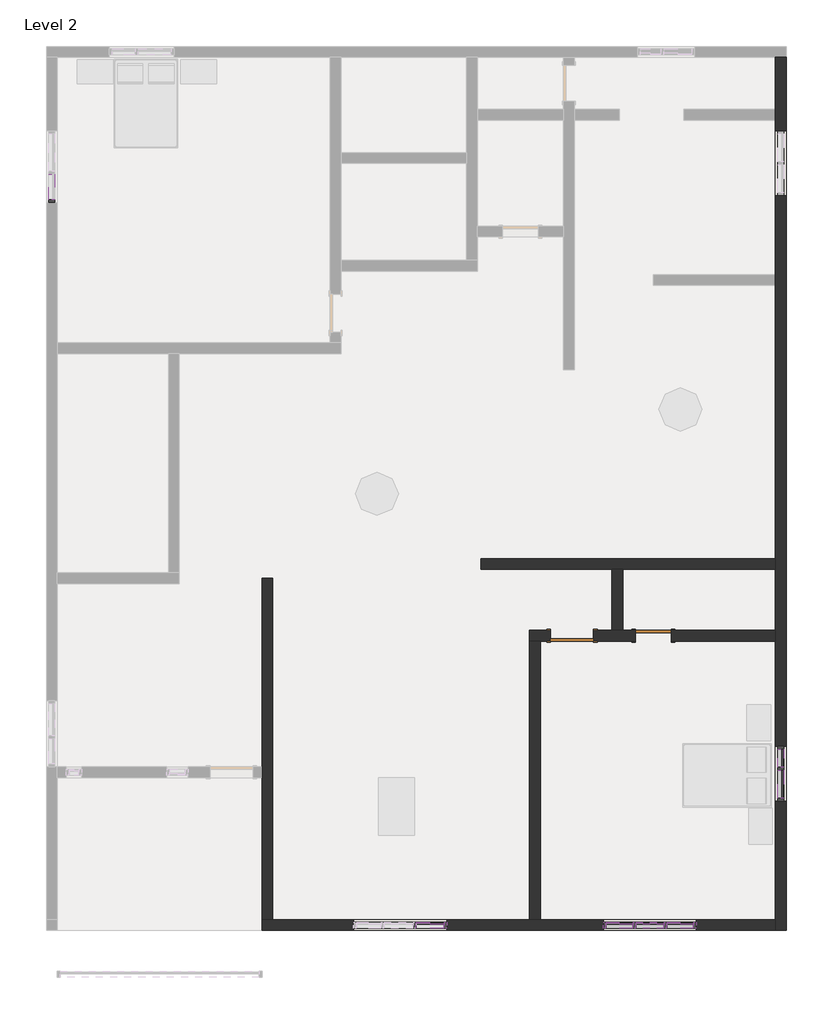
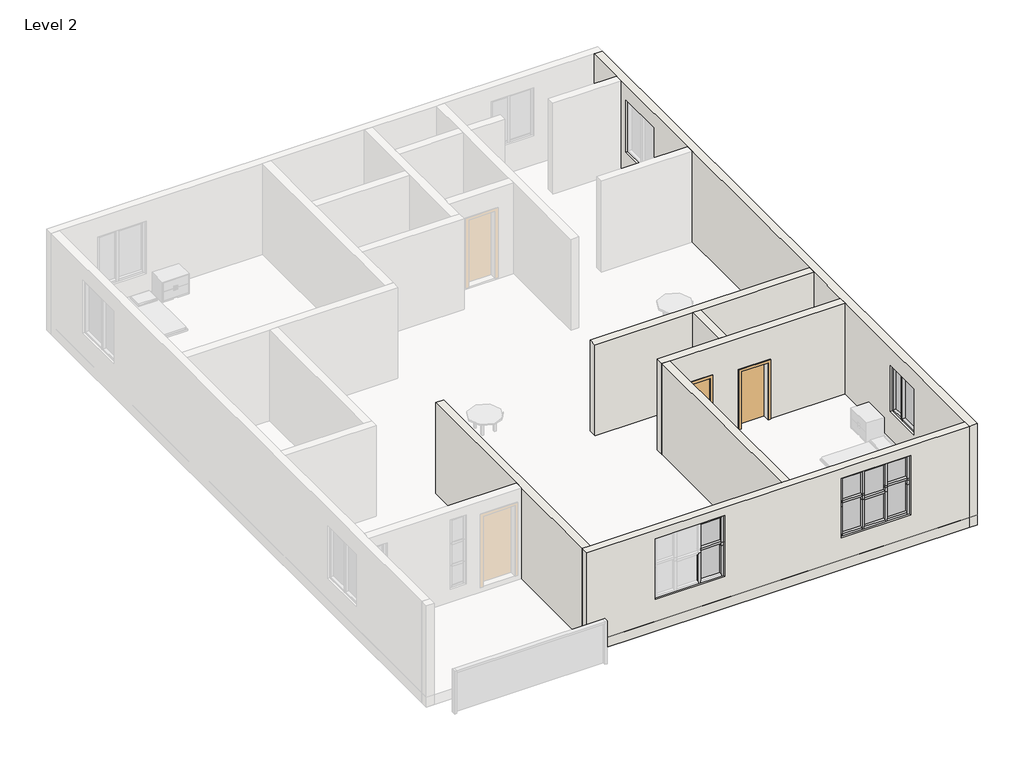
# One storey, part 2 of 3: 40 members, 10 plates, 7 walls, 2 doors.
"""IFC4 building model written with IfcOpenShell, lengths in millimetres."""

from ifc_helpers import new_model, si_unit, frame, origin, place, context, project, spatial, polyline, outline, extrude, faceted_brep, transform, mapped, element, save
from components import door_a1484949, door_0ca8825f, member_6f432376, member_6103f85b, member_a400357f, member_86293703, member_dffdf235, member_e5d39754, member_4dfd3f86, member_6a2a75bf, member_411778f3, member_a8e3eee7, member_06e32611, member_a86422a6, member_06be906d, member_67d1cd44, member_7190e7de, member_9cc26bde, member_6a93b315, member_fb13da3b, member_5b006e0e, member_8ea47e38, member_29dce480, member_81de2198, member_b315899a, system_panel_glazed_958ccbb4, system_panel_glazed_a29d5ab1, system_panel_glazed_48a86efd, system_panel_glazed_6d48a8a8, system_panel_glazed_893369a6, system_panel_glazed_ba2d6641, system_panel_glazed_82992491, system_panel_glazed_5721f284, system_panel_glazed_0c2a6c90, system_panel_glazed_e4ad360d

model = new_model("IFC4")

# Units and contexts
model_context = context("Model", 3, world=origin())
ifc_project = project(units=[si_unit("LENGTHUNIT", "METRE", prefix="MILLI")], contexts=[model_context])

# Site, building, storey
site = spatial("IfcSite", under=ifc_project)
building = spatial("IfcBuilding", under=site)
storey = spatial("IfcBuildingStorey", under=building, Name="Level 2", Elevation=3048.0)

# Doors
placement = place(None, origin())
door_shape = door_a1484949(model_context)
element("IfcDoor", 1, ObjectType="Single-Flush : 30\" x 80\"", at=placement, inside=storey, context=model_context, shape_type="MappedRepresentation", body=[
    mapped(door_shape, transform((-6207.9702714, -5339.3383903, 3048.0), x_axis=(1.0, 0.0, 0.0), y_axis=(0.0, 1.0, 0.0), z_axis=(0.0, 0.0, 1.0))),
])
door_2_shape = door_0ca8825f(model_context)
element("IfcDoor", 2, ObjectType="Single-Flush : 36\" x 84\"", at=placement, inside=storey, context=model_context, shape_type="MappedRepresentation", body=[
    mapped(door_2_shape, transform((-7935.1702714, -5339.3383903, 3048.0), x_axis=(-1.0, 0.0, 0.0), y_axis=(0.0, -1.0, 0.0), z_axis=(0.0, 0.0, 1.0))),
])

# Members
member_shape = member_6f432376(model_context)
element("IfcMember", 3, ObjectType="Rectangular Mullion : 2.5\" x 5\" rectangular", at=placement, inside=storey, context=model_context, shape_type="MappedRepresentation", body=[
    mapped(member_shape, transform((-6646.1202714, -11473.4383903, 5811.6646409), x_axis=(0.0, 0.0, 1.0), y_axis=(0.0, -1.0, 0.0), z_axis=(1.0, 0.0, 0.0))),
])
element("IfcMember", 4, ObjectType="Rectangular Mullion : 2.5\" x 5\" rectangular", at=placement, inside=storey, context=model_context, shape_type="MappedRepresentation", body=[
    mapped(member_shape, transform((-5357.0702714, -11473.4383903, 5811.6646409), x_axis=(0.0, 0.0, 1.0), y_axis=(0.0, -1.0, 0.0), z_axis=(1.0, 0.0, 0.0))),
])
element("IfcMember", 5, ObjectType="Rectangular Mullion : 2.5\" x 5\" rectangular", at=placement, inside=storey, context=model_context, shape_type="MappedRepresentation", body=[
    mapped(member_shape, transform((-5922.2202714, -11473.4383903, 4016.8568253), x_axis=(0.0, 0.0, -1.0), y_axis=(0.0, -1.0, 0.0), z_axis=(-1.0, 0.0, 0.0))),
])
element("IfcMember", 6, ObjectType="Rectangular Mullion : 2.5\" x 5\" rectangular", at=placement, inside=storey, context=model_context, shape_type="MappedRepresentation", body=[
    mapped(member_shape, transform((-7211.2702714, -11473.4383903, 4016.8568253), x_axis=(0.0, 0.0, -1.0), y_axis=(0.0, -1.0, 0.0), z_axis=(-1.0, 0.0, 0.0))),
])
member_2_shape = member_6103f85b(model_context)
element("IfcMember", 7, ObjectType="Rectangular Mullion : 2.5\" x 5\" rectangular", at=placement, inside=storey, context=model_context, shape_type="MappedRepresentation", body=[
    mapped(member_2_shape, transform((-6646.1202714, -11473.4383903, 5041.2607331), x_axis=(0.0, 0.0, 1.0), y_axis=(0.0, -1.0, 0.0), z_axis=(1.0, 0.0, 0.0))),
])
element("IfcMember", 8, ObjectType="Rectangular Mullion : 2.5\" x 5\" rectangular", at=placement, inside=storey, context=model_context, shape_type="MappedRepresentation", body=[
    mapped(member_2_shape, transform((-5357.0702714, -11473.4383903, 5092.0607331), x_axis=(0.0, 0.0, 1.0), y_axis=(0.0, -1.0, 0.0), z_axis=(1.0, 0.0, 0.0))),
])
member_3_shape = member_a400357f(model_context)
element("IfcMember", 9, ObjectType="Rectangular Mullion : 2.5\" x 5\" rectangular", at=placement, inside=storey, context=model_context, shape_type="MappedRepresentation", body=[
    mapped(member_3_shape, transform((-5985.7202714, -11473.4383903, 5811.6646409), x_axis=(0.0, 0.0, 1.0), y_axis=(0.0, -1.0, 0.0), z_axis=(1.0, 0.0, 0.0))),
])
element("IfcMember", 10, ObjectType="Rectangular Mullion : 2.5\" x 5\" rectangular", at=placement, inside=storey, context=model_context, shape_type="MappedRepresentation", body=[
    mapped(member_3_shape, transform((-6582.6202714, -11473.4383903, 4016.8568253), x_axis=(0.0, 0.0, -1.0), y_axis=(0.0, -1.0, 0.0), z_axis=(-1.0, 0.0, 0.0))),
])
member_4_shape = member_86293703(model_context)
element("IfcMember", 11, ObjectType="Rectangular Mullion : 2.5\" x 5\" rectangular", at=placement, inside=storey, context=model_context, shape_type="MappedRepresentation", body=[
    mapped(member_4_shape, transform((-5985.7202714, -11473.4383903, 4914.2607331), x_axis=(0.0, 0.0, 1.0), y_axis=(0.0, -1.0, 0.0), z_axis=(1.0, 0.0, 0.0))),
])
member_5_shape = member_dffdf235(model_context)
element("IfcMember", 12, ObjectType="Rectangular Mullion : 2.5\" x 5\" rectangular", at=placement, inside=storey, context=model_context, shape_type="MappedRepresentation", body=[
    mapped(member_5_shape, transform((-3502.8702714, -8126.9883903, 5563.9039141), x_axis=(0.0, 0.0, 1.0), y_axis=(-1.0, 0.0, 0.0), z_axis=(0.0, -1.0, 0.0))),
])
member_6_shape = member_e5d39754(model_context)
element("IfcMember", 13, ObjectType="Rectangular Mullion : 2.5\" x 5\" rectangular", at=placement, inside=storey, context=model_context, shape_type="MappedRepresentation", body=[
    mapped(member_6_shape, transform((-3502.8702714, -8781.0383903, 5563.9039141), x_axis=(0.0, 0.0, 1.0), y_axis=(-1.0, 0.0, 0.0), z_axis=(0.0, -1.0, 0.0))),
])
element("IfcMember", 14, ObjectType="Rectangular Mullion : 2.5\" x 5\" rectangular", at=placement, inside=storey, context=model_context, shape_type="MappedRepresentation", body=[
    mapped(member_6_shape, transform((-10652.9702714, -11473.4383903, 5845.1081495), x_axis=(0.0, 0.0, 1.0), y_axis=(0.0, -1.0, 0.0), z_axis=(1.0, 0.0, 0.0))),
])
member_7_shape = member_4dfd3f86(model_context)
element("IfcMember", 15, ObjectType="Rectangular Mullion : 2.5\" x 5\" rectangular", at=placement, inside=storey, context=model_context, shape_type="MappedRepresentation", body=[
    mapped(member_7_shape, transform((-3502.8702714, -8158.7383903, 4179.1199852), x_axis=(0.0, -1.0, 0.0), y_axis=(-1.0, 0.0, 0.0), z_axis=(0.0, 0.0, -1.0))),
])
element("IfcMember", 16, ObjectType="Rectangular Mullion : 2.5\" x 5\" rectangular", at=placement, inside=storey, context=model_context, shape_type="MappedRepresentation", body=[
    mapped(member_6_shape, transform((-3502.8702714, -8190.4883903, 4179.1199852), x_axis=(0.0, 0.0, -1.0), y_axis=(-1.0, 0.0, 0.0), z_axis=(0.0, 1.0, 0.0))),
])
element("IfcMember", 17, ObjectType="Rectangular Mullion : 2.5\" x 5\" rectangular", at=placement, inside=storey, context=model_context, shape_type="MappedRepresentation", body=[
    mapped(member_5_shape, transform((-3502.8702714, -7739.6383903, 4179.1199852), x_axis=(0.0, 0.0, -1.0), y_axis=(-1.0, 0.0, 0.0), z_axis=(0.0, 1.0, 0.0))),
])
member_8_shape = member_6a2a75bf(model_context)
element("IfcMember", 18, ObjectType="Rectangular Mullion : 2.5\" x 5\" rectangular", at=placement, inside=storey, context=model_context, shape_type="MappedRepresentation", body=[
    mapped(member_8_shape, transform((-3502.8702714, -7676.1383903, 5563.9039141), x_axis=(0.0, 1.0, 0.0), y_axis=(-1.0, 0.0, 0.0), z_axis=(0.0, 0.0, 1.0))),
])
element("IfcMember", 19, ObjectType="Rectangular Mullion : 2.5\" x 5\" rectangular", at=placement, inside=storey, context=model_context, shape_type="MappedRepresentation", body=[
    mapped(member_8_shape, transform((-3502.8702714, -8844.5383903, 4179.1199852), x_axis=(0.0, -1.0, 0.0), y_axis=(-1.0, 0.0, 0.0), z_axis=(0.0, 0.0, -1.0))),
])
member_9_shape = member_411778f3(model_context)
element("IfcMember", 20, ObjectType="Rectangular Mullion : 2.5\" x 5\" rectangular", at=placement, inside=storey, context=model_context, shape_type="MappedRepresentation", body=[
    mapped(member_9_shape, transform((-7274.7702714, -11473.4383903, 5811.6646409), x_axis=(-1.0, 0.0, 0.0), y_axis=(0.0, -1.0, 0.0), z_axis=(0.0, 0.0, 1.0))),
])
member_10_shape = member_a8e3eee7(model_context)
element("IfcMember", 21, ObjectType="Rectangular Mullion : 2.5\" x 5\" rectangular", at=placement, inside=storey, context=model_context, shape_type="MappedRepresentation", body=[
    mapped(member_10_shape, transform((-5293.5702714, -11473.4383903, 4914.2607331), x_axis=(1.0, 0.0, 0.0), y_axis=(0.0, -1.0, 0.0), z_axis=(0.0, 0.0, -1.0))),
])
member_11_shape = member_06e32611(model_context)
element("IfcMember", 22, ObjectType="Rectangular Mullion : 2.5\" x 5\" rectangular", at=placement, inside=storey, context=model_context, shape_type="MappedRepresentation", body=[
    mapped(member_11_shape, transform((-7274.7702714, -11473.4383903, 4914.2607331), x_axis=(-1.0, 0.0, 0.0), y_axis=(0.0, -1.0, 0.0), z_axis=(0.0, 0.0, 1.0))),
])
element("IfcMember", 23, ObjectType="Rectangular Mullion : 2.5\" x 5\" rectangular", at=placement, inside=storey, context=model_context, shape_type="MappedRepresentation", body=[
    mapped(member_11_shape, transform((-5293.5702714, -11473.4383903, 4016.8568253), x_axis=(1.0, 0.0, 0.0), y_axis=(0.0, -1.0, 0.0), z_axis=(0.0, 0.0, -1.0))),
])
member_12_shape = member_a86422a6(model_context)
element("IfcMember", 24, ObjectType="Rectangular Mullion : 2.5\" x 5\" rectangular", at=placement, inside=storey, context=model_context, shape_type="MappedRepresentation", body=[
    mapped(member_12_shape, transform((-6614.3702714, -11473.4383903, 5092.0607331), x_axis=(1.0, 0.0, 0.0), y_axis=(0.0, -1.0, 0.0), z_axis=(0.0, 0.0, -1.0))),
])
member_13_shape = member_06be906d(model_context)
element("IfcMember", 25, ObjectType="Rectangular Mullion : 2.5\" x 5\" rectangular", at=placement, inside=storey, context=model_context, shape_type="MappedRepresentation", body=[
    mapped(member_13_shape, transform((-6614.3702714, -11473.4383903, 5041.2607331), x_axis=(1.0, 0.0, 0.0), y_axis=(0.0, -1.0, 0.0), z_axis=(0.0, 0.0, -1.0))),
])
member_14_shape = member_67d1cd44(model_context)
element("IfcMember", 26, ObjectType="Rectangular Mullion : 2.5\" x 5\" rectangular", at=placement, inside=storey, context=model_context, shape_type="MappedRepresentation", body=[
    mapped(member_14_shape, transform((-7274.7702714, -11473.4383903, 5092.0607331), x_axis=(-1.0, 0.0, 0.0), y_axis=(0.0, -1.0, 0.0), z_axis=(0.0, 0.0, 1.0))),
])
element("IfcMember", 27, ObjectType="Rectangular Mullion : 2.5\" x 5\" rectangular", at=placement, inside=storey, context=model_context, shape_type="MappedRepresentation", body=[
    mapped(member_10_shape, transform((-7274.7702714, -11473.4383903, 5041.2607331), x_axis=(-1.0, 0.0, 0.0), y_axis=(0.0, -1.0, 0.0), z_axis=(0.0, 0.0, 1.0))),
])
member_15_shape = member_7190e7de(model_context)
element("IfcMember", 28, ObjectType="Rectangular Mullion : 2.5\" x 5\" rectangular", at=placement, inside=storey, context=model_context, shape_type="MappedRepresentation", body=[
    mapped(member_15_shape, transform((-5953.9702714, -11473.4383903, 4914.2607331), x_axis=(1.0, 0.0, 0.0), y_axis=(0.0, -1.0, 0.0), z_axis=(0.0, 0.0, -1.0))),
])
member_16_shape = member_9cc26bde(model_context)
element("IfcMember", 29, ObjectType="Rectangular Mullion : 2.5\" x 5\" rectangular", at=placement, inside=storey, context=model_context, shape_type="MappedRepresentation", body=[
    mapped(member_16_shape, transform((-5953.9702714, -11473.4383903, 4016.8568253), x_axis=(1.0, 0.0, 0.0), y_axis=(0.0, -1.0, 0.0), z_axis=(0.0, 0.0, -1.0))),
])
element("IfcMember", 30, ObjectType="Rectangular Mullion : 2.5\" x 5\" rectangular", at=placement, inside=storey, context=model_context, shape_type="MappedRepresentation", body=[
    mapped(member_16_shape, transform((-6614.3702714, -11473.4383903, 4016.8568253), x_axis=(1.0, 0.0, 0.0), y_axis=(0.0, -1.0, 0.0), z_axis=(0.0, 0.0, -1.0))),
])
element("IfcMember", 31, ObjectType="Rectangular Mullion : 2.5\" x 5\" rectangular", at=placement, inside=storey, context=model_context, shape_type="MappedRepresentation", body=[
    mapped(member_15_shape, transform((-6614.3702714, -11473.4383903, 4914.2607331), x_axis=(1.0, 0.0, 0.0), y_axis=(0.0, -1.0, 0.0), z_axis=(0.0, 0.0, -1.0))),
])
element("IfcMember", 32, ObjectType="Rectangular Mullion : 2.5\" x 5\" rectangular", at=placement, inside=storey, context=model_context, shape_type="MappedRepresentation", body=[
    mapped(member_12_shape, transform((-5953.9702714, -11473.4383903, 5092.0607331), x_axis=(1.0, 0.0, 0.0), y_axis=(0.0, -1.0, 0.0), z_axis=(0.0, 0.0, -1.0))),
])
element("IfcMember", 33, ObjectType="Rectangular Mullion : 2.5\" x 5\" rectangular", at=placement, inside=storey, context=model_context, shape_type="MappedRepresentation", body=[
    mapped(member_13_shape, transform((-5953.9702714, -11473.4383903, 5041.2607331), x_axis=(1.0, 0.0, 0.0), y_axis=(0.0, -1.0, 0.0), z_axis=(0.0, 0.0, -1.0))),
])
element("IfcMember", 34, ObjectType="Rectangular Mullion : 2.5\" x 5\" rectangular", at=placement, inside=storey, context=model_context, shape_type="MappedRepresentation", body=[
    mapped(member_9_shape, transform((-5293.5702714, -11473.4383903, 5092.0607331), x_axis=(1.0, 0.0, 0.0), y_axis=(0.0, -1.0, 0.0), z_axis=(0.0, 0.0, -1.0))),
])
element("IfcMember", 35, ObjectType="Rectangular Mullion : 2.5\" x 5\" rectangular", at=placement, inside=storey, context=model_context, shape_type="MappedRepresentation", body=[
    mapped(member_14_shape, transform((-5293.5702714, -11473.4383903, 5041.2607331), x_axis=(1.0, 0.0, 0.0), y_axis=(0.0, -1.0, 0.0), z_axis=(0.0, 0.0, -1.0))),
])
member_17_shape = member_6a93b315(model_context)
element("IfcMember", 36, ObjectType="Rectangular Mullion : 2.5\" x 5\" rectangular", at=placement, inside=storey, context=model_context, shape_type="MappedRepresentation", body=[
    mapped(member_17_shape, transform((-10589.4702714, -11473.4383903, 4012.7558847), x_axis=(1.0, 0.0, 0.0), y_axis=(0.0, -1.0, 0.0), z_axis=(0.0, 0.0, -1.0))),
])
member_18_shape = member_fb13da3b(model_context)
element("IfcMember", 37, ObjectType="Rectangular Mullion : 2.5\" x 5\" rectangular", at=placement, inside=storey, context=model_context, shape_type="MappedRepresentation", body=[
    mapped(member_18_shape, transform((-10589.4702714, -11473.4383903, 4928.9320171), x_axis=(1.0, 0.0, 0.0), y_axis=(0.0, -1.0, 0.0), z_axis=(0.0, 0.0, -1.0))),
])
member_19_shape = member_5b006e0e(model_context)
element("IfcMember", 38, ObjectType="Rectangular Mullion : 2.5\" x 5\" rectangular", at=placement, inside=storey, context=model_context, shape_type="MappedRepresentation", body=[
    mapped(member_19_shape, transform((-10589.4702714, -11473.4383903, 5030.5320171), x_axis=(1.0, 0.0, 0.0), y_axis=(0.0, -1.0, 0.0), z_axis=(0.0, 0.0, -1.0))),
])
member_20_shape = member_8ea47e38(model_context)
element("IfcMember", 39, ObjectType="Rectangular Mullion : 2.5\" x 5\" rectangular", at=placement, inside=storey, context=model_context, shape_type="MappedRepresentation", body=[
    mapped(member_20_shape, transform((-11275.2702714, -11473.4383903, 4012.7558847), x_axis=(1.0, 0.0, 0.0), y_axis=(0.0, -1.0, 0.0), z_axis=(0.0, 0.0, -1.0))),
])
member_21_shape = member_29dce480(model_context)
element("IfcMember", 40, ObjectType="Rectangular Mullion : 2.5\" x 5\" rectangular", at=placement, inside=storey, context=model_context, shape_type="MappedRepresentation", body=[
    mapped(member_21_shape, transform((-10652.9702714, -11473.4383903, 5030.5320171), x_axis=(0.0, 0.0, 1.0), y_axis=(0.0, -1.0, 0.0), z_axis=(1.0, 0.0, 0.0))),
])
member_22_shape = member_81de2198(model_context)
element("IfcMember", 41, ObjectType="Rectangular Mullion : 2.5\" x 5\" rectangular", at=placement, inside=storey, context=model_context, shape_type="MappedRepresentation", body=[
    mapped(member_22_shape, transform((-18971.4702714, 3906.2616097, 5636.3811186), x_axis=(0.0, 0.0, 1.0), y_axis=(-1.0, 0.0, 0.0), z_axis=(0.0, -1.0, 0.0))),
])
member_23_shape = member_b315899a(model_context)
element("IfcMember", 42, ObjectType="Rectangular Mullion : 2.5\" x 5\" rectangular", at=placement, inside=storey, context=model_context, shape_type="MappedRepresentation", body=[
    mapped(member_23_shape, transform((-18971.4702714, 3842.7616097, 4041.7365925), x_axis=(0.0, -1.0, 0.0), y_axis=(-1.0, 0.0, 0.0), z_axis=(0.0, 0.0, -1.0))),
])

# Plates
system_panel_glazed_shape = system_panel_glazed_958ccbb4(model_context)
element("IfcPlate", 43, ObjectType="System Panel : Glazed", at=placement, inside=storey, context=model_context, shape_type="MappedRepresentation", body=[
    mapped(system_panel_glazed_shape, transform((-3502.8702714, -7933.3133903, 4242.6199852), x_axis=(0.0, -1.0, 0.0), y_axis=(1.0, 0.0, 0.0), z_axis=(0.0, 0.0, 1.0))),
])
system_panel_glazed_2_shape = system_panel_glazed_a29d5ab1(model_context)
element("IfcPlate", 44, ObjectType="System Panel : Glazed", at=placement, inside=storey, context=model_context, shape_type="MappedRepresentation", body=[
    mapped(system_panel_glazed_2_shape, transform((-3502.8702714, -8485.7633903, 4242.6199852), x_axis=(0.0, -1.0, 0.0), y_axis=(1.0, 0.0, 0.0), z_axis=(0.0, 0.0, 1.0))),
])
system_panel_glazed_3_shape = system_panel_glazed_48a86efd(model_context)
element("IfcPlate", 45, ObjectType="System Panel : Glazed", at=placement, inside=storey, context=model_context, shape_type="MappedRepresentation", body=[
    mapped(system_panel_glazed_3_shape, transform((-6928.6952714, -11473.4383903, 4080.3568253), x_axis=(1.0, 0.0, 0.0), y_axis=(0.0, 1.0, 0.0), z_axis=(0.0, 0.0, 1.0))),
])
system_panel_glazed_4_shape = system_panel_glazed_6d48a8a8(model_context)
element("IfcPlate", 46, ObjectType="System Panel : Glazed", at=placement, inside=storey, context=model_context, shape_type="MappedRepresentation", body=[
    mapped(system_panel_glazed_4_shape, transform((-6928.6952714, -11473.4383903, 5073.0107331), x_axis=(1.0, 0.0, 0.0), y_axis=(0.0, 1.0, 0.0), z_axis=(0.0, 0.0, 1.0))),
])
system_panel_glazed_5_shape = system_panel_glazed_893369a6(model_context)
element("IfcPlate", 47, ObjectType="System Panel : Glazed", at=placement, inside=storey, context=model_context, shape_type="MappedRepresentation", body=[
    mapped(system_panel_glazed_5_shape, transform((-6284.1702714, -11473.4383903, 4080.3568253), x_axis=(1.0, 0.0, 0.0), y_axis=(0.0, 1.0, 0.0), z_axis=(0.0, 0.0, 1.0))),
])
system_panel_glazed_6_shape = system_panel_glazed_ba2d6641(model_context)
element("IfcPlate", 48, ObjectType="System Panel : Glazed", at=placement, inside=storey, context=model_context, shape_type="MappedRepresentation", body=[
    mapped(system_panel_glazed_6_shape, transform((-6284.1702714, -11473.4383903, 4946.0107331), x_axis=(1.0, 0.0, 0.0), y_axis=(0.0, 1.0, 0.0), z_axis=(0.0, 0.0, 1.0))),
])
system_panel_glazed_7_shape = system_panel_glazed_82992491(model_context)
element("IfcPlate", 49, ObjectType="System Panel : Glazed", at=placement, inside=storey, context=model_context, shape_type="MappedRepresentation", body=[
    mapped(system_panel_glazed_7_shape, transform((-5639.6452714, -11473.4383903, 4080.3568253), x_axis=(1.0, 0.0, 0.0), y_axis=(0.0, 1.0, 0.0), z_axis=(0.0, 0.0, 1.0))),
])
system_panel_glazed_8_shape = system_panel_glazed_5721f284(model_context)
element("IfcPlate", 50, ObjectType="System Panel : Glazed", at=placement, inside=storey, context=model_context, shape_type="MappedRepresentation", body=[
    mapped(system_panel_glazed_8_shape, transform((-5639.6452714, -11473.4383903, 5123.8107331), x_axis=(1.0, 0.0, 0.0), y_axis=(0.0, 1.0, 0.0), z_axis=(0.0, 0.0, 1.0))),
])
system_panel_glazed_9_shape = system_panel_glazed_0c2a6c90(model_context)
element("IfcPlate", 51, ObjectType="System Panel : Glazed", at=placement, inside=storey, context=model_context, shape_type="MappedRepresentation", body=[
    mapped(system_panel_glazed_9_shape, transform((-10948.2452714, -11473.4383903, 4076.2558847), x_axis=(1.0, 0.0, 0.0), y_axis=(0.0, 1.0, 0.0), z_axis=(0.0, 0.0, 1.0))),
])
system_panel_glazed_10_shape = system_panel_glazed_e4ad360d(model_context)
element("IfcPlate", 52, ObjectType="System Panel : Glazed", at=placement, inside=storey, context=model_context, shape_type="MappedRepresentation", body=[
    mapped(system_panel_glazed_10_shape, transform((-10948.2452714, -11473.4383903, 5062.2820171), x_axis=(1.0, 0.0, 0.0), y_axis=(0.0, 1.0, 0.0), z_axis=(0.0, 0.0, 1.0))),
])

# Walls
element("IfcWall", 53, ObjectType="9\"", at=placement, inside=storey, context=model_context, shape_type="Brep", body=[
    faceted_brep([(-3617.1702714, 6928.8616097, 3048.0), (-3617.1702714, 5823.9616097, 3048.0), (-3617.1702714, 5595.3616097, 3048.0), (-3617.1702714, 2318.7616097, 3048.0), (-3617.1702714, 2090.1616097, 3048.0), (-3617.1702714, -3701.0383903, 3048.0), (-3617.1702714, -3929.6383903, 3048.0), (-3617.1702714, -5225.0383903, 3048.0), (-3617.1702714, -5453.6383903, 3048.0), (-3617.1702714, -11359.1383903, 3048.0), (-3617.1702714, -11587.7383903, 3048.0), (-3617.1702714, -11587.7383903, 6096.0), (-3617.1702714, -11359.1383903, 6096.0), (-3617.1702714, -5453.6383903, 6096.0), (-3617.1702714, -5225.0383903, 6096.0), (-3617.1702714, -3929.6383903, 6096.0), (-3617.1702714, -3701.0383903, 6096.0), (-3617.1702714, 2090.1616097, 6096.0), (-3617.1702714, 2318.7616097, 6096.0), (-3617.1702714, 5595.3616097, 6096.0), (-3617.1702714, 5823.9616097, 6096.0), (-3617.1702714, 6928.8616097, 6096.0), (-3617.1702714, -7676.1383903, 4179.1199852), (-3617.1702714, -7676.1383903, 5563.9039141), (-3617.1702714, -8844.5383903, 5563.9039141), (-3617.1702714, -8844.5383903, 4179.1199852), (-3617.1702714, 5366.7616097, 4078.2335743), (-3617.1702714, 5366.7616097, 5644.9656178), (-3617.1702714, 3995.1616097, 5644.9656178), (-3617.1702714, 3995.1616097, 4078.2335743), (-3388.5702714, -11587.7383903, 3048.0), (-3388.5702714, 6928.8616097, 3048.0), (-3388.5702714, 6928.8616097, 6096.0), (-3388.5702714, -11587.7383903, 6096.0), (-3388.5702714, -7676.1383903, 5563.9039141), (-3388.5702714, -7676.1383903, 4179.1199852), (-3388.5702714, -8844.5383903, 4179.1199852), (-3388.5702714, -8844.5383903, 5563.9039141), (-3388.5702714, 5366.7616097, 5644.9656178), (-3388.5702714, 5366.7616097, 4078.2335743), (-3388.5702714, 3995.1616097, 4078.2335743), (-3388.5702714, 3995.1616097, 5644.9656178)], [[[0, 1, 2, 3, 4, 5, 6, 7, 8, 9, 10, 11, 12, 13, 14, 15, 16, 17, 18, 19, 20, 21], [22, 23, 24, 25], [26, 27, 28, 29]], [[30, 31, 32, 33], [34, 35, 36, 37], [38, 39, 40, 41]], [[10, 9, 8, 7, 6, 5, 4, 3, 2, 1, 0, 31, 30]], [[21, 20, 19, 18, 17, 16, 15, 14, 13, 12, 11, 33, 32]], [[0, 21, 32, 31]], [[11, 10, 30, 33]], [[34, 23, 22, 35]], [[23, 34, 37, 24]], [[24, 37, 36, 25]], [[35, 22, 25, 36]], [[26, 39, 38, 27]], [[27, 38, 41, 28]], [[28, 41, 40, 29]], [[39, 26, 29, 40]]]),
])
element("IfcWall", 54, ObjectType="9\"", at=placement, inside=storey, context=model_context, shape_type="Brep", body=[
    faceted_brep([(-3617.1702714, -11359.1383903, 3048.0), (-8608.2702714, -11359.1383903, 3048.0), (-8836.8702714, -11359.1383903, 3048.0), (-14285.1702714, -11359.1383903, 3048.0), (-14513.7702714, -11359.1383903, 3048.0), (-14513.7702714, -11359.1383903, 6096.0), (-14285.1702714, -11359.1383903, 6096.0), (-8836.8702714, -11359.1383903, 6096.0), (-8608.2702714, -11359.1383903, 6096.0), (-3617.1702714, -11359.1383903, 6096.0), (-12570.6702714, -11359.1383903, 5845.1081495), (-12570.6702714, -11359.1383903, 4012.7558847), (-10589.4702714, -11359.1383903, 4012.7558847), (-10589.4702714, -11359.1383903, 5845.1081495), (-7274.7702714, -11359.1383903, 5811.6646409), (-7274.7702714, -11359.1383903, 4016.8568253), (-5293.5702714, -11359.1383903, 4016.8568253), (-5293.5702714, -11359.1383903, 5811.6646409), (-14513.7702714, -11587.7383903, 3048.0), (-3617.1702714, -11587.7383903, 3048.0), (-3617.1702714, -11587.7383903, 6096.0), (-14513.7702714, -11587.7383903, 6096.0), (-12570.6702714, -11587.7383903, 4012.7558847), (-12570.6702714, -11587.7383903, 5845.1081495), (-10589.4702714, -11587.7383903, 5845.1081495), (-10589.4702714, -11587.7383903, 4012.7558847), (-7274.7702714, -11587.7383903, 4016.8568253), (-7274.7702714, -11587.7383903, 5811.6646409), (-5293.5702714, -11587.7383903, 5811.6646409), (-5293.5702714, -11587.7383903, 4016.8568253)], [[[0, 1, 2, 3, 4, 5, 6, 7, 8, 9], [10, 11, 12, 13], [14, 15, 16, 17]], [[18, 19, 20, 21], [22, 23, 24, 25], [26, 27, 28, 29]], [[4, 3, 2, 1, 0, 19, 18]], [[5, 4, 18, 21]], [[9, 8, 7, 6, 5, 21, 20]], [[0, 9, 20, 19]], [[22, 11, 10, 23]], [[23, 10, 13, 24]], [[24, 13, 12, 25]], [[11, 22, 25, 12]], [[14, 27, 26, 15]], [[27, 14, 17, 28]], [[28, 17, 16, 29]], [[15, 26, 29, 16]]]),
])
element("IfcWall", 55, ObjectType="9\"", at=placement, inside=storey, context=model_context, shape_type="Brep", body=[
    faceted_brep([(-14513.7702714, -4120.1383903, 3048.0), (-14513.7702714, -8120.6383903, 3048.0), (-14513.7702714, -8349.2383903, 3048.0), (-14513.7702714, -11359.1383903, 3048.0), (-14513.7702714, -11359.1383903, 6096.0), (-14513.7702714, -8349.2383903, 6096.0), (-14513.7702714, -8120.6383903, 6096.0), (-14513.7702714, -4120.1383903, 6096.0), (-14285.1702714, -4120.1383903, 3048.0), (-14285.1702714, -4120.1383903, 6096.0), (-14285.1702714, -11359.1383903, 6096.0), (-14285.1702714, -11359.1383903, 3048.0)], [[[0, 1, 2, 3, 4, 5, 6, 7]], [[8, 9, 10, 11]], [[3, 2, 1, 0, 8, 11]], [[7, 6, 5, 4, 10, 9]], [[0, 7, 9, 8]], [[4, 3, 11, 10]]]),
])
element("IfcWall", 56, ObjectType="9\"", at=placement, inside=storey, context=model_context, shape_type="SweptSolid", body=[
    extrude(outline(polyline([(-8836.8702714, -11359.1383903), (-8836.8702714, -5453.6383903), (-8608.2702714, -5453.6383903), (-8608.2702714, -11359.1383903), (-8836.8702714, -11359.1383903)])), frame((0.0, 0.0, 3048.0), z_axis=(0.0, 0.0, 1.0), x_axis=(1.0, 0.0, 0.0)), (0.0, 0.0, 1.0), 3048.0),
])
element("IfcWall", 57, ObjectType="9\"", at=placement, inside=storey, context=model_context, shape_type="Brep", body=[
    faceted_brep([(-3617.1702714, -3701.0383903, 3048.0), (-9865.5702714, -3701.0383903, 3048.0), (-9865.5702714, -3701.0383903, 6096.0), (-3617.1702714, -3701.0383903, 6096.0), (-3617.1702714, -3929.6383903, 3048.0), (-3617.1702714, -3929.6383903, 6096.0), (-6855.6702714, -3929.6383903, 6096.0), (-7084.2702714, -3929.6383903, 6096.0), (-9865.5702714, -3929.6383903, 6096.0), (-9865.5702714, -3929.6383903, 3048.0), (-7084.2702714, -3929.6383903, 3048.0), (-6855.6702714, -3929.6383903, 3048.0)], [[[0, 1, 2, 3]], [[4, 5, 6, 7, 8, 9, 10, 11]], [[1, 0, 4, 11, 10, 9]], [[2, 1, 9, 8]], [[3, 2, 8, 7, 6, 5]], [[0, 3, 5, 4]]]),
])
element("IfcWall", 58, ObjectType="9\"", at=placement, inside=storey, context=model_context, shape_type="SweptSolid", body=[
    extrude(outline(polyline([(-7084.2702714, -5225.0383903), (-7084.2702714, -3929.6383903), (-6855.6702714, -3929.6383903), (-6855.6702714, -5225.0383903), (-7084.2702714, -5225.0383903)])), frame((0.0, 0.0, 3048.0), z_axis=(0.0, 0.0, 1.0), x_axis=(1.0, 0.0, 0.0)), (0.0, 0.0, 1.0), 3048.0),
])
element("IfcWall", 59, ObjectType="9\"", at=placement, inside=storey, context=model_context, shape_type="Brep", body=[
    faceted_brep([(-5826.9702714, -5453.6383903, 5080.0), (-5826.9702714, -5453.6383903, 3048.0), (-3617.1702714, -5453.6383903, 3048.0), (-3617.1702714, -5453.6383903, 6096.0), (-8608.2702714, -5453.6383903, 6096.0), (-8836.8702714, -5453.6383903, 6096.0), (-8836.8702714, -5453.6383903, 3048.0), (-8608.2702714, -5453.6383903, 3048.0), (-8392.3702714, -5453.6383903, 3048.0), (-8392.3702714, -5453.6383903, 5181.6), (-7477.9702714, -5453.6383903, 5181.6), (-7477.9702714, -5453.6383903, 3048.0), (-6588.9702714, -5453.6383903, 3048.0), (-6588.9702714, -5453.6383903, 5080.0), (-3617.1702714, -5225.0383903, 3048.0), (-5826.9702714, -5225.0383903, 3048.0), (-5826.9702714, -5225.0383903, 5080.0), (-6588.9702714, -5225.0383903, 5080.0), (-6588.9702714, -5225.0383903, 3048.0), (-6855.6702714, -5225.0383903, 3048.0), (-7084.2702714, -5225.0383903, 3048.0), (-7477.9702714, -5225.0383903, 3048.0), (-7477.9702714, -5225.0383903, 5181.6), (-8392.3702714, -5225.0383903, 5181.6), (-8392.3702714, -5225.0383903, 3048.0), (-8836.8702714, -5225.0383903, 3048.0), (-8836.8702714, -5225.0383903, 6096.0), (-7084.2702714, -5225.0383903, 6096.0), (-6855.6702714, -5225.0383903, 6096.0), (-3617.1702714, -5225.0383903, 6096.0)], [[[0, 1, 2, 3, 4, 5, 6, 7, 8, 9, 10, 11, 12, 13]], [[14, 15, 16, 17, 18, 19, 20, 21, 22, 23, 24, 25, 26, 27, 28, 29]], [[25, 24, 8, 7, 6]], [[12, 11, 21, 20, 19, 18]], [[2, 1, 15, 14]], [[5, 4, 3, 29, 28, 27, 26]], [[6, 5, 26, 25]], [[3, 2, 14, 29]], [[9, 8, 24, 23]], [[10, 9, 23, 22]], [[11, 10, 22, 21]], [[16, 15, 1, 0]], [[17, 16, 0, 13]], [[18, 17, 13, 12]]]),
])

save(model, "model.ifc")

# Revit data of these elements
# Type "Single-Flush : 30\" x 80\""
#   Type Mark = "5"
#   Construction Type Id = "MDOOR"
#   Assembly Code = "C1020"
#   Analytic Construction = "Metal"
#   Thickness = 0' - 2"
#   Heat Transfer Coefficient (U) = 0.651978 BTU/(h·ft²·°F)
#   Height = 6' - 8"
#   Trim Projection Ext = 0' - 1"
#   Trim Projection Int = 0' - 1"
#   Trim Width = 0' - 3"
#   Width = 2' - 6"
#   Define Thermal Properties by = 1
#   Define Thermal Properties by = 1
#   Door Material = Door - Panel
#   Frame Material = Door - Frame
#   Visual Light Transmittance = 0
#   Solar Heat Gain Coefficient = 0
#   Function = (empty or 0)
#   Wall Closure = (empty or 0)
# Type "Single-Flush : 36\" x 84\""
#   Type Mark = "1"
#   Construction Type Id = "MDOOR"
#   Assembly Code = "C1020"
#   Analytic Construction = "Metal"
#   Thickness = 0' - 2"
#   Heat Transfer Coefficient (U) = 0.651978 BTU/(h·ft²·°F)
#   Height = 7' - 0"
#   Trim Projection Ext = 0' - 1"
#   Trim Projection Int = 0' - 1"
#   Trim Width = 0' - 3"
#   Width = 3' - 0"
#   Define Thermal Properties by = 1
#   Define Thermal Properties by = 1
#   Door Material = Door - Panel
#   Frame Material = Door - Frame
#   Visual Light Transmittance = 0
#   Solar Heat Gain Coefficient = 0
#   Function = (empty or 0)
#   Wall Closure = (empty or 0)
# Type "Rectangular Mullion : 2.5\" x 5\" rectangular"
#   built-in parameter 1007304 = 0.416667 (stored number, unit not read)
#   built-in parameter 1007301 = 0.104167 (stored number, unit not read)
#   built-in parameter 1007300 = 0.104167 (stored number, unit not read)
# Type "System Panel : Glazed"
#   Construction Type Id = "GSP4R"
#   Analytic Construction = "1/8 in Pilkington single glazing"
#   Visual Light Transmittance = 0.9
#   Solar Heat Gain Coefficient = 0.86
#   Heat Transfer Coefficient (U) = 1.18115 BTU/(h·ft²·°F)
#   Define Thermal Properties by = 1
# Type "9\""
#   Assembly Code = "B2010"
#   Layers, outside or top first: 0' - 9" no material (function 1)
# Element 1 (IfcDoor, "Single-Flush : 30\" x 80\"")
#   Phase Created = New Construction
#   Materials on its faces: "Door - Frame", "Door - Panel"
# Element 2 (IfcDoor, "Single-Flush : 36\" x 84\"")
#   Phase Created = New Construction
#   Materials on its faces: "Door - Frame", "Door - Panel"
# Elements 3, 4, 5, 6, 7, 8, 9, 10, 11, 12, 13, 14, 15, 16, 17, 18, 19, 20, 21, 22, 23, 24, 25, 26, 27, 28, 29, 30, 31, 32, 33, 34, 35, 36, 37, 38, 39, 40, 41, 42 (IfcMember, "Rectangular Mullion : 2.5\" x 5\" rectangular")
#   Phase Created = New Construction
#   Materials on its faces: "Aluminum"
# Elements 43, 44, 45, 46, 47, 48, 49, 50, 51, 52 (IfcPlate, "System Panel : Glazed")
#   Phase Created = New Construction
#   Materials on its faces: "Glass"
# Elements 53, 54, 55, 56, 57, 58, 59 (IfcWall, "9\"")
#   Top Offset = 0' - 0"
#   Base Offset = 0' - 0"
#   Unconnected Height = 10' - 0"
#   wall height = 10' - 0"
#   Phase Created = New Construction
#   Base Constraint = Level 2
#   Materials on its faces: "Default Wall"
# Materials
#   "Door - Panel": class "Wood", colour RGB 210 159 95, transparency 0, Cost = 0
#   "Door - Frame": colour RGB 118 70 51, transparency 0, Cost = 0
#   "Aluminum": class "Metal", colour RGB 247 247 247, transparency 0, Description = "Aluminum 6061", Cost = 0
#   "Glass": class "Glass", colour RGB 0 128 192, transparency 0.75, Description = "Soda Lime Glass", Cost = 0
#   "Default Wall": colour RGB 128 128 128, transparency 0, Cost = 0
